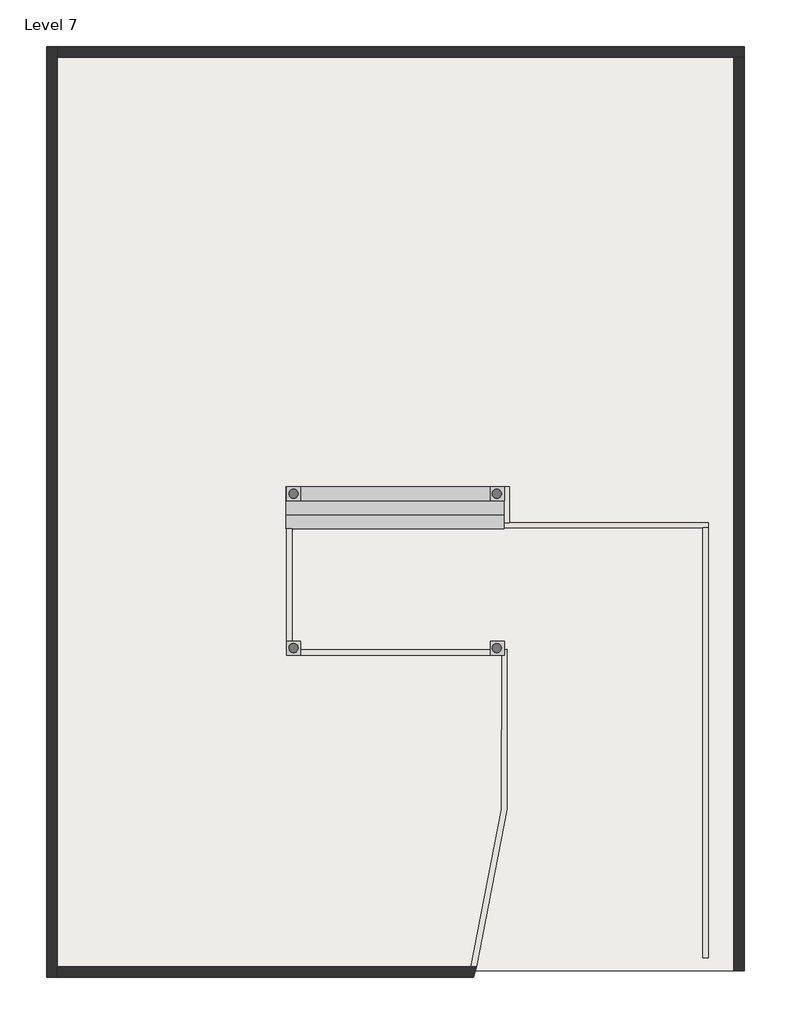
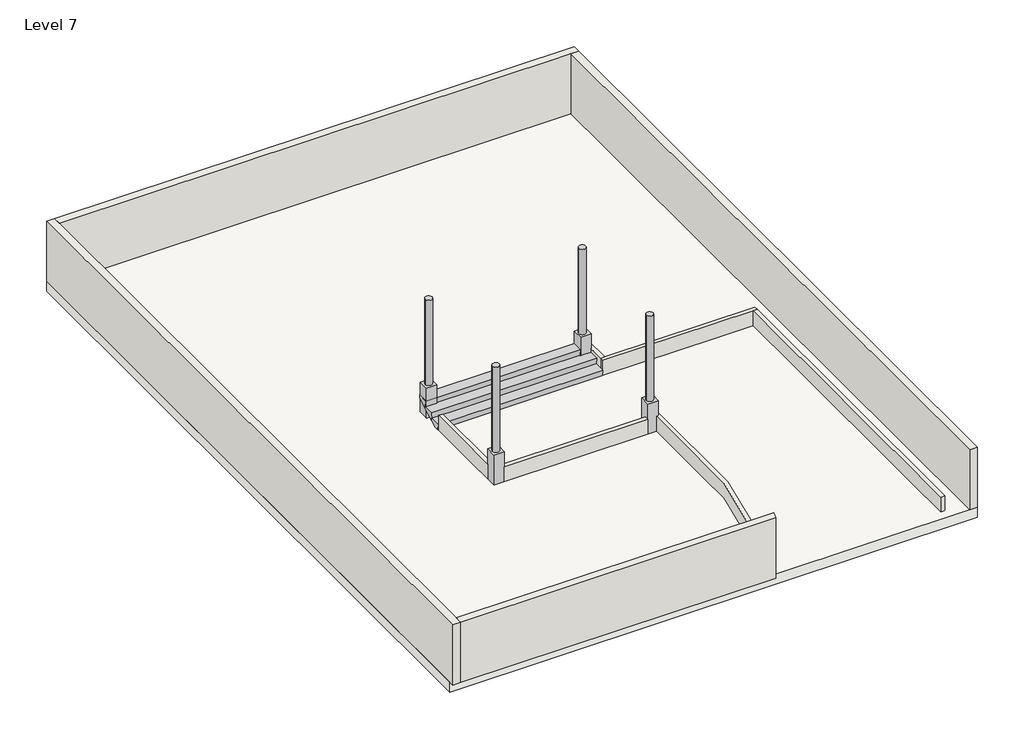
# One storey, incomplete: 10 walls, 1 proxy, 1 slab, 1 stair flight.
"""IFC4 building model written with IfcOpenShell, lengths in millimetres."""

from ifc_helpers import new_model, si_unit, point, frame, frame_2d, origin, place, context, project, spatial, polyline, circle_curve, trimmed, segment, composite_curve, outline, extrude, faceted_brep, transform, mapped, element, save
from ifc_brep_helpers import plane_surface, cylinder_surface, advanced_brep
from components import generic_models_3_generic_models_3_02764364

model = new_model("IFC4")

# Units and contexts
model_context = context("Model", 3, world=origin())
ifc_project = project(units=[si_unit("LENGTHUNIT", "METRE", prefix="MILLI")], contexts=[model_context])

# Site, building, storey
site = spatial("IfcSite", under=ifc_project)
building = spatial("IfcBuilding", under=site)
storey = spatial("IfcBuildingStorey", under=building, Name="Level 7", Elevation=-609.6)

# Proxy
placement = place(None, origin())
generic_models_3_generic_models_3_shape = generic_models_3_generic_models_3_02764364(model_context)
element("IfcBuildingElementProxy", 1, Name="Generic Models 3 : Generic Models 3", ObjectType="Generic Models 3 : Generic Models 3", at=placement, inside=storey, context=model_context, shape_type="MappedRepresentation", body=[
    mapped(generic_models_3_generic_models_3_shape, transform((0.0, 0.0, 0.0), x_axis=(1.0, 0.0, 0.0), y_axis=(0.0, 1.0, 0.0), z_axis=(0.0, 0.0, 1.0))),
])

# Slab
element("IfcSlab", 2, ObjectType="Generic - 12\"", at=placement, inside=storey, context=model_context, shape_type="SweptSolid", body=[
    extrude(outline(polyline([(-5272.8088298, 13059.3124124), (-5272.8088298, -7019.3875876), (-20440.5593474, -7019.3875876), (-20440.5593474, 13059.3124124), (-5272.8088298, 13059.3124124)])), frame((0.0, 0.0, -914.4), z_axis=(0.0, 0.0, 1.0), x_axis=(1.0, 0.0, 0.0)), (0.0, 0.0, 1.0), 304.8),
])

# Stair flight
element("IfcStairFlight", 3, ObjectType="3/4\" Nosing", at=placement, inside=storey, context=model_context, shape_type="Brep", body=[
    faceted_brep([(-15233.3556236, 2582.4153836, -434.34), (-10497.8531829, 2582.4153836, -434.34), (-10497.8531829, 2906.7256859, -434.34), (-15233.3556236, 2906.7256859, -434.34), (-15233.3556236, 2906.7256859, -507.5615483), (-15233.3556236, 2728.9995156, -609.6), (-15233.3556236, 2601.4653836, -609.6), (-10497.8531829, 2601.4653836, -609.6), (-10497.8531829, 2728.9995156, -609.6), (-10497.8531829, 2906.7256859, -507.5615483), (-15233.3556236, 2887.6756859, -259.08), (-10497.8531829, 2887.6756859, -259.08), (-10497.8531829, 3211.9859881, -259.08), (-15233.3556236, 3211.9859881, -259.08), (-15233.3556236, 3211.9859881, -332.3015483), (-10497.8531829, 3211.9859881, -332.3015483), (-15233.3556236, 3192.9359881, -83.82), (-10497.8531829, 3192.9359881, -83.82), (-10497.8531829, 3498.1962903, -83.82), (-15233.3556236, 3498.1962903, -83.82), (-15233.3556236, 3498.1962903, -167.9787811), (-10497.8531829, 3498.1962903, -167.9787811)], [[[0, 1, 2, 3]], [[0, 3, 4, 5, 6]], [[2, 1, 7, 8, 9]], [[10, 11, 12, 13]], [[10, 13, 14, 4, 3]], [[12, 11, 2, 9, 15]], [[1, 0, 6, 7]], [[3, 2, 11, 10]], [[16, 17, 18, 19]], [[16, 19, 20, 14, 13]], [[18, 17, 12, 15, 21]], [[19, 18, 21, 20]], [[13, 12, 17, 16]], [[7, 6, 5, 8]], [[8, 5, 4, 14, 20, 21, 15, 9]]]),
])

# Walls
element("IfcWall", 4, ObjectType="4.5\"", at=placement, inside=storey, context=model_context, shape_type="SweptSolid", body=[
    extrude(outline(composite_curve([segment(polyline([(-10540.8741466, -46.4616519), (-10427.0864726, -35.6516918)]), True, "CONTINUOUS"), segment(trimmed(circle_curve(frame_2d((-28690.0081554, -1770.650289)), 18345.15), [point((-10427.0864726, -35.6516918))], [point((-11088.5904327, -6941.2037097))], False, "CARTESIAN"), True, "CONTINUOUS"), segment(polyline([(-11088.5904327, -6941.2037097), (-11207.7523213, -6941.2037097)]), True, "CONTINUOUS"), segment(trimmed(circle_curve(frame_2d((-28690.0081554, -1770.650289)), 18230.85), [point((-11207.7523213, -6941.2037097))], [point((-10540.8741466, -46.4616519))], True, "CARTESIAN"), True, "CONTINUOUS")], self_intersect=False)), frame((0.0, 0.0, -609.6), z_axis=(0.0, 0.0, 1.0), x_axis=(1.0, 0.0, 0.0)), (0.0, 0.0, 1.0), 457.2),
])
element("IfcWall", 5, ObjectType="4.5\"", at=placement, inside=storey, context=model_context, shape_type="Brep", body=[
    faceted_brep([(-10483.9803096, 2599.5819165, -609.6), (-6168.1588298, 2599.5819165, -609.6), (-6053.8588298, 2599.5819165, -609.6), (-6053.8588298, 2599.5819165, -152.4), (-6168.1588298, 2599.5819165, -152.4), (-10483.9803096, 2599.5819165, -152.4), (-10483.9803096, 2713.8819165, -609.6), (-10483.9803096, 2713.8819165, -152.4), (-10369.6803096, 2713.8819165, -152.4), (-6053.8588298, 2713.8819165, -152.4), (-6053.8588298, 2713.8819165, -609.6), (-10369.6803096, 2713.8819165, -609.6)], [[[0, 1, 2, 3, 4, 5]], [[6, 7, 8, 9, 10, 11]], [[2, 1, 0, 6, 11, 10]], [[5, 4, 3, 9, 8, 7]], [[3, 2, 10, 9]], [[0, 5, 7, 6]]]),
])
element("IfcWall", 6, ObjectType="4.5\"", at=placement, inside=storey, context=model_context, shape_type="SweptSolid", body=[
    extrude(outline(polyline([(-6053.8588298, 2599.5819165), (-6053.8588298, -6738.0037097), (-6168.1588298, -6738.0037097), (-6168.1588298, 2599.5819165), (-6053.8588298, 2599.5819165)])), frame((0.0, 0.0, -609.6), z_axis=(0.0, 0.0, 1.0), x_axis=(1.0, 0.0, 0.0)), (0.0, 0.0, 1.0), 457.2),
])
element("IfcWall", 7, ObjectType="4.5\"", at=placement, inside=storey, context=model_context, shape_type="SweptSolid", body=[
    extrude(outline(polyline([(-14916.206326, -49.642926), (-10789.2406119, -49.642926), (-10789.2406119, -163.942926), (-14916.206326, -163.942926), (-14916.206326, -49.642926)])), frame((0.0, 0.0, -609.6), z_axis=(0.0, 0.0, 1.0), x_axis=(1.0, 0.0, 0.0)), (0.0, 0.0, 1.0), 457.2),
])
element("IfcWall", 8, ObjectType="4.5\"", at=placement, inside=storey, context=model_context, shape_type="SweptSolid", body=[
    extrude(outline(polyline([(-15105.1827503, 2579.7173763), (-15105.1827503, 141.3173763), (-15219.4827503, 141.3173763), (-15219.4827503, 2579.7173763), (-15105.1827503, 2579.7173763)])), frame((0.0, 0.0, -609.6), z_axis=(0.0, 0.0, 1.0), x_axis=(1.0, 0.0, 0.0)), (0.0, 0.0, 1.0), 457.2),
])
element("IfcWall", 9, ObjectType="4.5\"", at=placement, inside=storey, context=model_context, shape_type="SweptSolid", body=[
    extrude(outline(polyline([(-10369.6803096, 3495.212945), (-10369.6803096, 2713.8819165), (-10483.9803096, 2713.8819165), (-10483.9803096, 3495.212945), (-10369.6803096, 3495.212945)])), frame((0.0, 0.0, -609.6), z_axis=(0.0, 0.0, 1.0), x_axis=(1.0, 0.0, 0.0)), (0.0, 0.0, 1.0), 457.2),
])
element("IfcWall", 10, ObjectType="9\"", at=placement, inside=storey, context=model_context, shape_type="Brep", body=[
    faceted_brep([(-20211.9593474, -7169.8037097, -609.6), (-20211.9593474, -6941.2037097, -609.6), (-20211.9593474, 12830.7124124, -609.6), (-20211.9593474, 13059.3124124, -609.6), (-20211.9593474, 13059.3124124, 1219.2), (-20211.9593474, 12830.7124124, 1219.2), (-20211.9593474, -6941.2037097, 1219.2), (-20211.9593474, -7169.8037097, 1219.2), (-20440.5593474, -7169.8037097, -609.6), (-20440.5593474, -7169.8037097, 1219.2), (-20440.5593474, 13059.3124124, 1219.2), (-20440.5593474, 13059.3124124, -609.6)], [[[0, 1, 2, 3, 4, 5, 6, 7]], [[8, 9, 10, 11]], [[3, 2, 1, 0, 8, 11]], [[7, 6, 5, 4, 10, 9]], [[0, 7, 9, 8]], [[4, 3, 11, 10]]]),
])
element("IfcWall", 11, ObjectType="9\"", at=placement, inside=storey, context=model_context, shape_type="Brep", body=[
    faceted_brep([(-20211.9593474, 12830.7124124, -609.6), (-5501.4088298, 12830.7124124, -609.6), (-5272.8088298, 12830.7124124, -609.6), (-5272.8088298, 12830.7124124, 1219.2), (-5501.4088298, 12830.7124124, 1219.2), (-20211.9593474, 12830.7124124, 1219.2), (-20211.9593474, 13059.3124124, -609.6), (-20211.9593474, 13059.3124124, 1219.2), (-5272.8088298, 13059.3124124, 1219.2), (-5272.8088298, 13059.3124124, -609.6)], [[[0, 1, 2, 3, 4, 5]], [[6, 7, 8, 9]], [[2, 1, 0, 6, 9]], [[5, 4, 3, 8, 7]], [[3, 2, 9, 8]], [[0, 5, 7, 6]]]),
])
element("IfcWall", 12, ObjectType="9\"", at=placement, inside=storey, context=model_context, shape_type="SweptSolid", body=[
    extrude(outline(polyline([(-5501.4088298, -7019.3875876), (-5501.4088298, 12830.7124124), (-5272.8088298, 12830.7124124), (-5272.8088298, -7019.3875876), (-5501.4088298, -7019.3875876)])), frame((0.0, 0.0, -609.6), z_axis=(0.0, 0.0, 1.0), x_axis=(1.0, 0.0, 0.0)), (0.0, 0.0, 1.0), 1828.8),
])
element("IfcWall", 13, ObjectType="9\"", at=placement, inside=storey, context=model_context, shape_type="AdvancedBrep", body=[
    advanced_brep(
    [(-11088.5904327, -6941.2037097, -609.6), (-11207.7523213, -6941.2037097, -609.6), (-20211.9593474, -6941.2037097, -609.6), (-20211.9593474, -6941.2037097, 1219.2), (-11088.5904327, -6941.2037097, 1219.2), (-11088.5904327, -6941.2037097, -152.4), (-11157.3622951, -7169.8037097, -609.6), (-11157.3622951, -7169.8037097, 1219.2), (-20211.9593474, -7169.8037097, 1219.2), (-20211.9593474, -7169.8037097, -609.6)],
    [
        (0, 1),
        (1, 2),
        (2, 3),
        (3, 4),
        (4, 5),
        (5, 0),
        (6, 7),
        (7, 8),
        (8, 9),
        (9, 6),
        (0, 6, circle_curve(frame((-28690.0081554, -1770.650289, -609.6), z_axis=(0.0, 0.0, -1.0), x_axis=(1.0, 0.0, 0.0)), 18345.15)),
        (9, 2),
        (3, 8),
        (7, 4, circle_curve(frame((-28690.0081554, -1770.650289, 1219.2), z_axis=(0.0, 0.0, 1.0), x_axis=(1.0, 0.0, 0.0)), 18345.15)),
    ],
    [
        plane_surface(frame((-15982.6335059, -6941.2037097, -609.6), z_axis=(0.0, 1.0, 0.0), x_axis=(-1.0, 0.0, 0.0))),
        plane_surface(frame((-15982.6335059, -7169.8037097, -609.6), z_axis=(0.0, -1.0, 0.0), x_axis=(1.0, 0.0, 0.0))),
        plane_surface(frame((-11182.2593474, -6941.2037097, -609.6), z_axis=(0.0, 0.0, -1.0), x_axis=(0.0, -1.0, 0.0))),
        plane_surface(frame((-20326.2593474, -6941.2037097, 1219.2), z_axis=(0.0, 0.0, 1.0), x_axis=(0.0, -1.0, 0.0))),
        plane_surface(frame((-20211.9593474, 8867.0121312, -609.6), z_axis=(-1.0, 0.0, 0.0), x_axis=(0.0, 1.0, 0.0))),
        cylinder_surface(frame((-28690.0081554, -1770.650289, -609.6), z_axis=(0.0, 0.0, 1.0), x_axis=(1.0, 0.0, 0.0)), 18345.15),
    ],
    [
        (0, [[1, 2, 3, 4, 5, 6]]),
        (1, [[7, 8, 9, 10]]),
        (2, [[-2, -1, 11, -10, 12]]),
        (3, [[-4, 13, -8, 14]]),
        (4, [[-3, -12, -9, -13]]),
        (5, [[-6, -5, -14, -7, -11]]),
    ],
),
])

save(model, "model.ifc")

# Revit data of these elements
# Type "Generic - 12\""
#   Assembly Code = "B1010"
#   Function = 0
#   Layers, outside or top first: 1' - 0" no material (function 1)
# Type "4.5\""
#   Assembly Code = "B2010"
#   Layers, outside or top first: 0' - 4 1/2" no material (function 1)
# Type "9\""
#   Assembly Code = "B2010"
#   Layers, outside or top first: 0' - 9" no material (function 1)
# Element 1 (IfcBuildingElementProxy, "Generic Models 3 : Generic Models 3")
#   Phase Created = New Construction
# Element 2 (IfcSlab, "Generic - 12\"")
#   Height Offset From Level = 0' - 0"
#   Phase Created = New Construction
#   Materials on its faces: "Default Floor"
# Element 3 (IfcStairFlight, "3/4\" Nosing")
#   Phase Created = New Construction
#   Materials on its faces: "Concrete, Cast-in-Place gray"
# Element 4 (IfcWall, "4.5\"")
#   Top Offset = 10' - 0"
#   Base Offset = 0' - 0"
#   Unconnected Height = 1' - 6"
#   wall height = 1' - 6"
#   Phase Created = New Construction
#   Materials on its faces: "Default Wall"
# Elements 5, 6, 7, 8, 9 (IfcWall, "4.5\"")
#   Top Offset = 10' - 0"
#   Base Offset = 0' - 0"
#   Unconnected Height = 1' - 6"
#   wall height = 1' - 6"
#   Phase Created = New Construction
#   Base Constraint = Level 7
#   Materials on its faces: "Default Wall"
# Elements 10, 11, 12, 13 (IfcWall, "9\"")
#   Top Offset = 10' - 0"
#   Base Offset = 0' - 0"
#   Unconnected Height = 6' - 0"
#   wall height = 6' - 0"
#   Phase Created = New Construction
#   Base Constraint = Level 7
#   Materials on its faces: "Default Wall"
# Materials
#   "Default Floor": colour RGB 128 128 128, transparency 0, Cost = 0
#   "Concrete, Cast-in-Place gray": class "Concrete", colour RGB 192 192 192, transparency 0, Description = "Cast-in-place concrete", Cost = 0
#   "Default Wall": colour RGB 128 128 128, transparency 0, Cost = 0
